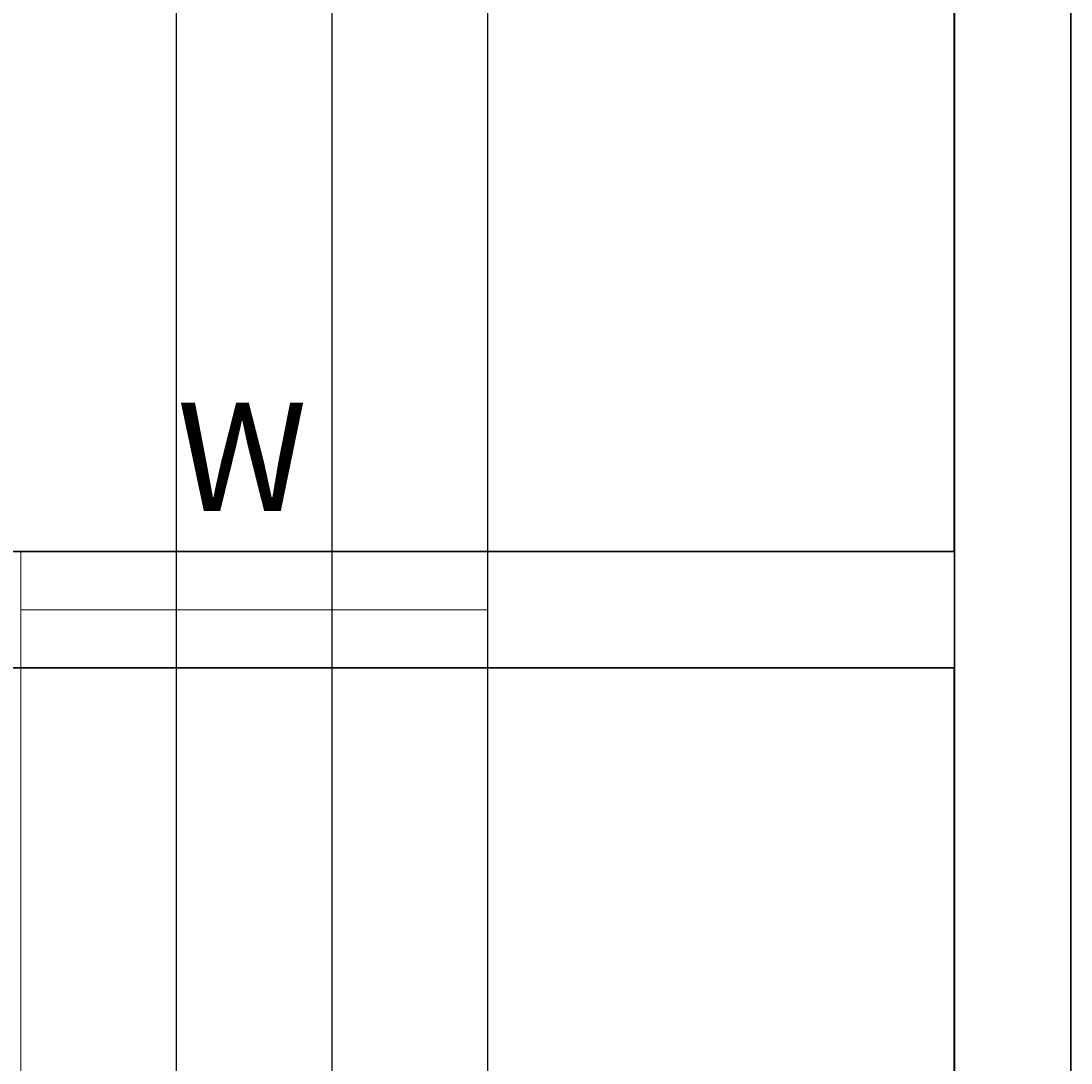
# Model space of a CAD drawing. Units: feet. Extents: x 1654 to 2985, y 1348 to 2230.
# Tile 45 of 53: x 2713 to 2794, y 1712 to 1792. Entities that reach past the tile are written whole.
import ezdxf

# ---------------------------------------------------------------- set-up
doc = ezdxf.new("R2010")
doc.units = ezdxf.units.FT
for name, color, linetype, lineweight in [('A-ANNO-DIMS', 2, 'Continuous', 18), ('A-ANNO-TEXT', 7, 'Continuous', 18), ('A-FLOR-STRS', 7, 'Continuous', 18), ('A-GLAZ', 4, 'Continuous', 18), ('A-WALL', 7, 'Continuous', 35)]:
    doc.layers.add(name, color=color, linetype=linetype, lineweight=lineweight)
doc.styles.get("Standard").update_dxf_attribs({"font": 'arial.ttf'})
doc.dimstyles.get("Standard").update_dxf_attribs({"dimtxt": 0.18, "dimasz": 0.18, "dimexe": 0.18, "dimexo": 0.0625, "dimgap": 0.09, "dimtad": 0, "dimtih": 1, "dimtoh": 1, "dimdec": 4, "dimzin": 0, "dimdsep": 46, "dimtxsty": 'Standard', "dimcen": 0.09, "dimadec": 0, "dimazin": 0, "dimtfac": 1, "dimtdec": 4, "dimtofl": 0, "dimtmove": 0, "dimatfit": 3, "dimfxl": 1, "dimtolj": 1, "dimtzin": 0, "dimarcsym": 0})

# ---------------------------------------------------------------- blocks, each defined once
blk = doc.blocks.new('STAIR-RETURN')
for p, q in [((0, 186), (0, 135)), ((36, 186), (36, 0)), ((0, 177), (0, 135)), ((12, 177), (12, 135)), ((12, 177), (12, 135)), ((24, 177), (24, 135)), ((24, 177), (24, 135))]:
    blk.add_line(p, q)
blk = doc.blocks.new('*D82')
at = {"layer": 'A-ANNO-DIMS', "color": 0, "lineweight": -2, "transparency": 16777216}
for p, q in [((2652.706, 2039.192), (2652.706, 1490.625)), ((2784.706, 2039.192), (2784.706, 1490.625)), ((2652.886, 1490.805), (2718.426, 1490.805)), ((2784.526, 1490.805), (2718.985, 1490.805))]:
    blk.add_line(p, q, dxfattribs=at)
at = {"layer": 'A-ANNO-DIMS', "color": 0, "transparency": 16777216}
for points in [[(2652.886, 1490.835), (2652.886, 1490.775), (2652.706, 1490.805)], [(2784.526, 1490.835), (2784.526, 1490.775), (2784.706, 1490.805)]]:
    blk.add_solid(points, dxfattribs=at)
at = {"layer": 'Defpoints', "color": 0, "transparency": 16777216}
for p in [(2652.706, 2039.255), (2784.706, 2039.255), (2784.706, 1490.805)]:
    blk.add_point(p, dxfattribs=at)
at = {"layer": 'A-ANNO-DIMS', "color": 0, "transparency": 16777216, "insert": (2718.706, 1490.805), "char_height": 0.18, "attachment_point": 5}
blk.add_mtext('\\A1;132', dxfattribs=at)
blk = doc.blocks.new('*D86')
at = {"layer": 'A-ANNO-DIMS', "color": 0, "lineweight": -2, "transparency": 16777216}
for p, q in [((2748.706, 1616.317), (2748.706, 2149.885)), ((2784.706, 1607.317), (2784.706, 2149.885)), ((2748.886, 2149.705), (2766.487, 2149.705)), ((2784.526, 2149.705), (2766.925, 2149.705))]:
    blk.add_line(p, q, dxfattribs=at)
at = {"layer": 'A-ANNO-DIMS', "color": 0, "transparency": 16777216}
for points in [[(2748.886, 2149.735), (2748.886, 2149.675), (2748.706, 2149.705)], [(2784.526, 2149.735), (2784.526, 2149.675), (2784.706, 2149.705)]]:
    blk.add_solid(points, dxfattribs=at)
at = {"layer": 'Defpoints', "color": 0, "transparency": 16777216}
for p in [(2784.706, 2149.705), (2748.706, 1616.255), (2784.706, 1607.255)]:
    blk.add_point(p, dxfattribs=at)
at = {"layer": 'A-ANNO-DIMS', "color": 0, "transparency": 16777216, "insert": (2766.706, 2149.705), "char_height": 0.18, "attachment_point": 5}
blk.add_mtext('\\A1;36', dxfattribs=at)
blk = doc.blocks.new('*D87')
at = {"layer": 'A-ANNO-DIMS', "color": 0, "lineweight": -2, "transparency": 16777216}
for p, q in [((2724.706, 1565.317), (2724.706, 2149.885)), ((2736.706, 1565.317), (2736.706, 2149.885)), ((2724.886, 2149.705), (2730.496, 2149.705)), ((2736.526, 2149.705), (2730.915, 2149.705))]:
    blk.add_line(p, q, dxfattribs=at)
at = {"layer": 'A-ANNO-DIMS', "color": 0, "transparency": 16777216}
for points in [[(2724.886, 2149.735), (2724.886, 2149.675), (2724.706, 2149.705)], [(2736.526, 2149.735), (2736.526, 2149.675), (2736.706, 2149.705)]]:
    blk.add_solid(points, dxfattribs=at)
at = {"layer": 'Defpoints', "color": 0, "transparency": 16777216}
for p in [(2736.706, 2149.705), (2724.706, 1565.255), (2736.706, 1565.255)]:
    blk.add_point(p, dxfattribs=at)
at = {"layer": 'A-ANNO-DIMS', "color": 0, "transparency": 16777216, "insert": (2730.706, 2149.705), "char_height": 0.18, "attachment_point": 5}
blk.add_mtext('\\A1;12', dxfattribs=at)

msp = doc.modelspace()

# ---------------------------------------------------------------- linework, layer by layer
at = {"layer": 'A-GLAZ'}
msp.add_line((2748.7058, 1746.7549), (2712.7058, 1746.7549), dxfattribs=at)
at = {"layer": 'A-WALL'}
for p, q in [((2793.7058, 2117.2549), (2793.7058, 1742.2549)), ((2784.7058, 1886.2549), (2784.7058, 1751.2549)), ((2793.7058, 1886.2549), (2793.7058, 1523.2549)), ((2784.7058, 1751.2549), (2702.7058, 1751.2549)), ((2784.7058, 1742.2549), (2702.7058, 1742.2549)), ((2784.7058, 1742.2549), (2784.7058, 1565.2549))]:
    msp.add_line(p, q, dxfattribs=at)

# ---------------------------------------------------------------- block references
at = {"layer": 'A-FLOR-STRS'}
msp.add_blockref('STAIR-RETURN', (2712.7054, 1565.255), dxfattribs=at)

# ---------------------------------------------------------------- texts
at = {"layer": 'A-ANNO-TEXT'}
msp.add_text('W', height=8.3811, dxfattribs=at).set_placement((2724.7422, 1754.3563))

# ---------------------------------------------------------------- dimensions: what is measured, and where the dimension line sits
at = {"layer": 'A-ANNO-DIMS'}
for base, p1, p2, picture, middle in [((2736.7058, 2149.7049), (2724.7058, 1565.2549), (2736.7058, 1565.2549), '*D87', (2730.7058, 2149.7049)), ((2784.7058, 2149.7049), (2748.7058, 1616.2549), (2784.7058, 1607.2549), '*D86', (2766.7058, 2149.7049)), ((2784.7058, 1490.8049), (2652.7058, 2039.2549), (2784.7058, 2039.2549), '*D82', (2718.7058, 1490.8049))]:
    dim = msp.add_linear_dim(base=base, p1=p1, p2=p2, dimstyle='Standard', override={"dimdec": 0, "dimlfac": 1, "dimrnd": 0, "dimzin": 0, "dimdsep": 46, "dimlunit": 2}, dxfattribs=at)
    dim.commit()
    dim.dimension.update_dxf_attribs({"geometry": picture, "text_midpoint": middle})

doc.saveas('drawing.dxf')
